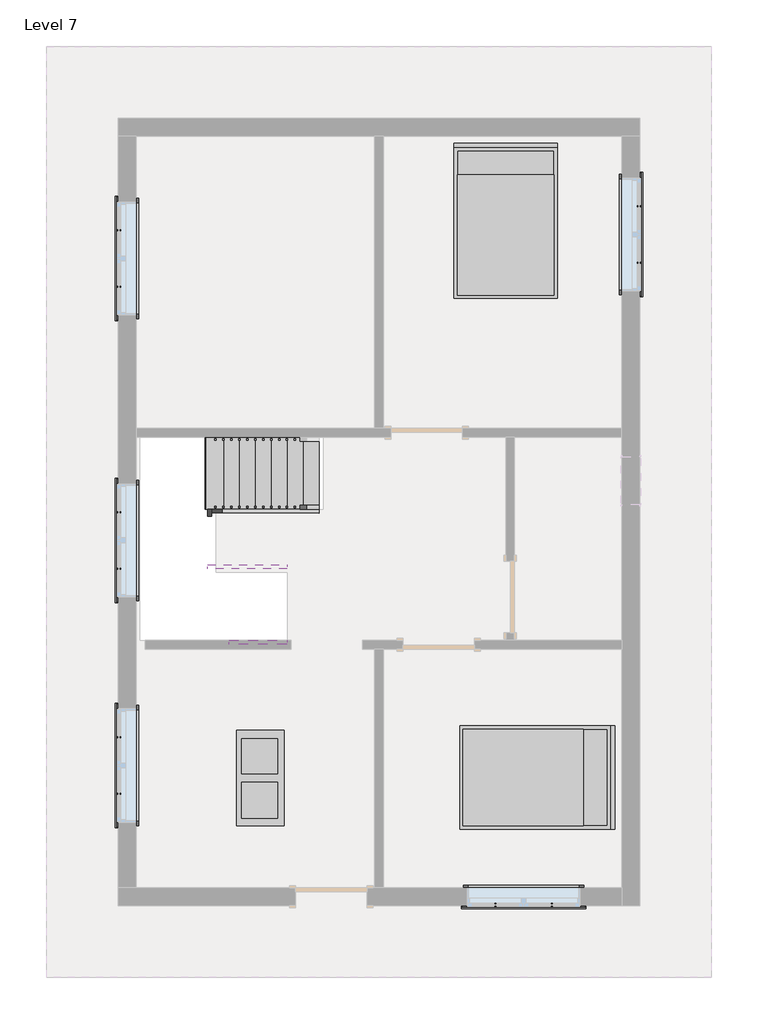
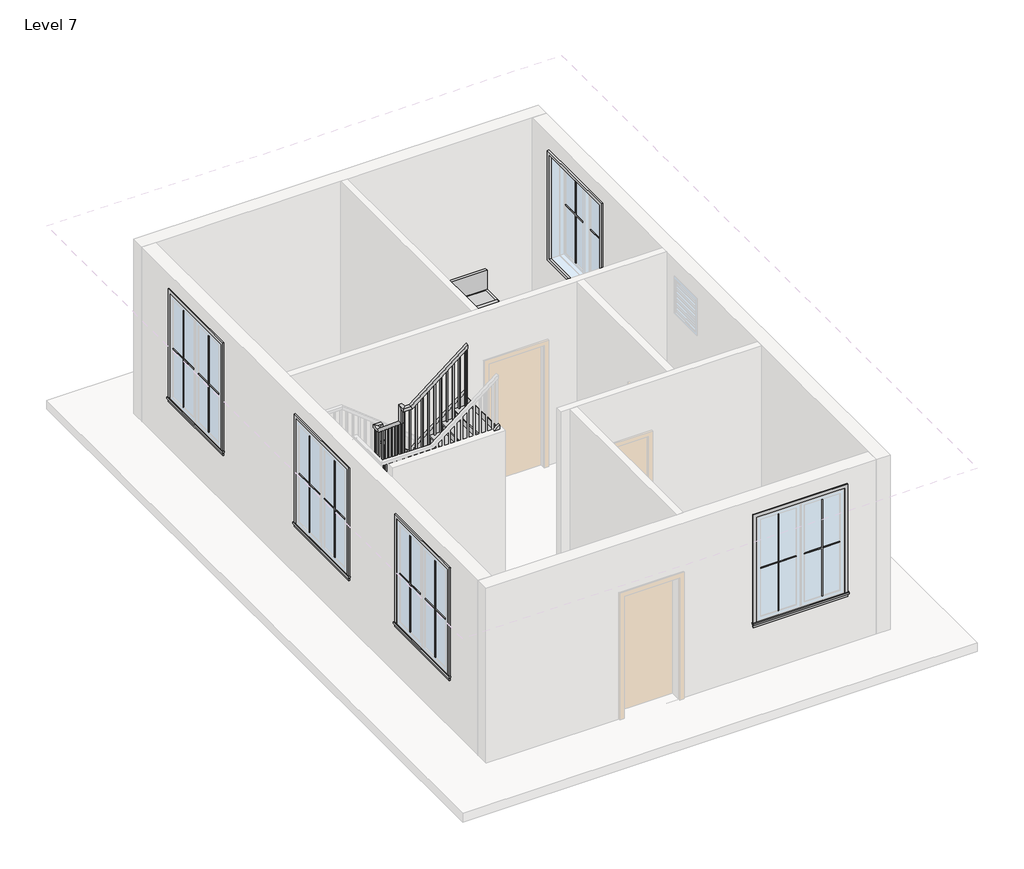
# One storey, part 2 of 2: 21 proxies, 5 members, 2 furniture elements, 1 railing, 1 stair flight.
"""IFC4 building model written with IfcOpenShell, lengths in millimetres."""

from ifc_helpers import new_model, si_unit, frame, origin, place, context, project, spatial, polyline, outline, extrude, faceted_brep, transform, mapped, element, save
from components import muntin_pattern_2x2_muntin_pattern_2x2_bff912c5, muntin_pattern_2x2_muntin_pattern_2x2_c2194282, trim_window_exterior_flat_with_sill_e04b3088, trim_window_interior_flat_picture_frame_2a7685fe, coffee_table_with_brass_mullions_11320_coffee_table_with_5962bef7, bed_17739_bed_17739_15c61121, stair_flight_dc8f8b64

model = new_model("IFC4")

# Units and contexts
model_context = context("Model", 3, world=origin())
ifc_project = project(units=[si_unit("LENGTHUNIT", "METRE", prefix="MILLI")], contexts=[model_context])

# Site, building, storey
site = spatial("IfcSite", under=ifc_project)
building = spatial("IfcBuilding", under=site)
storey = spatial("IfcBuildingStorey", under=building, Name="Level 7", Elevation=16002.0)

# Proxies
placement = place(None, origin())
muntin_pattern_2x2_muntin_pattern_2x2_shape = muntin_pattern_2x2_muntin_pattern_2x2_bff912c5(model_context)
element("IfcBuildingElementProxy", 1, Name="Muntin Pattern_2x2 : Muntin Pattern_2x2", ObjectType="Muntin Pattern_2x2 : Muntin Pattern_2x2", at=placement, inside=storey, context=model_context, shape_type="MappedRepresentation", body=[
    mapped(muntin_pattern_2x2_muntin_pattern_2x2_shape, transform((-626.5715247, -5050.1430046, 16986.25), x_axis=(-1.0, 0.0, 0.0), y_axis=(0.0, -1.0, 0.0), z_axis=(0.0, 0.0, 1.0))),
])
element("IfcBuildingElementProxy", 2, Name="Muntin Pattern_2x2 : Muntin Pattern_2x2", ObjectType="Muntin Pattern_2x2 : Muntin Pattern_2x2", at=placement, inside=storey, context=model_context, shape_type="MappedRepresentation", body=[
    mapped(muntin_pattern_2x2_muntin_pattern_2x2_shape, transform((-6159.0090247, -3629.3305046, 16986.25), x_axis=(0.0, 1.0, 0.0), y_axis=(-1.0, 0.0, 0.0), z_axis=(0.0, 0.0, 1.0))),
])
element("IfcBuildingElementProxy", 3, Name="Muntin Pattern_2x2 : Muntin Pattern_2x2", ObjectType="Muntin Pattern_2x2 : Muntin Pattern_2x2", at=placement, inside=storey, context=model_context, shape_type="MappedRepresentation", body=[
    mapped(muntin_pattern_2x2_muntin_pattern_2x2_shape, transform((489.4409753, 3873.1944954, 16986.25), x_axis=(0.0, -1.0, 0.0), y_axis=(1.0, 0.0, 0.0), z_axis=(0.0, 0.0, 1.0))),
])
element("IfcBuildingElementProxy", 4, Name="Muntin Pattern_2x2 : Muntin Pattern_2x2", ObjectType="Muntin Pattern_2x2 : Muntin Pattern_2x2", at=placement, inside=storey, context=model_context, shape_type="MappedRepresentation", body=[
    mapped(muntin_pattern_2x2_muntin_pattern_2x2_shape, transform((-6159.0090247, 2847.6694954, 16986.25), x_axis=(0.0, 1.0, 0.0), y_axis=(-1.0, 0.0, 0.0), z_axis=(0.0, 0.0, 1.0))),
])
element("IfcBuildingElementProxy", 5, Name="Muntin Pattern_2x2 : Muntin Pattern_2x2", ObjectType="Muntin Pattern_2x2 : Muntin Pattern_2x2", at=placement, inside=storey, context=model_context, shape_type="MappedRepresentation", body=[
    mapped(muntin_pattern_2x2_muntin_pattern_2x2_shape, transform((-6159.0090247, -752.7805046, 16986.25), x_axis=(0.0, 1.0, 0.0), y_axis=(-1.0, 0.0, 0.0), z_axis=(0.0, 0.0, 1.0))),
])
muntin_pattern_2x2_muntin_pattern_2x2_2_shape = muntin_pattern_2x2_muntin_pattern_2x2_c2194282(model_context)
element("IfcBuildingElementProxy", 6, Name="Muntin Pattern_2x2 : Muntin Pattern_2x2", ObjectType="Muntin Pattern_2x2 : Muntin Pattern_2x2", at=placement, inside=storey, context=model_context, shape_type="MappedRepresentation", body=[
    mapped(muntin_pattern_2x2_muntin_pattern_2x2_2_shape, transform((-1347.2965247, -5050.1430046, 16986.25), x_axis=(1.0, 0.0, 0.0), y_axis=(0.0, 1.0, 0.0), z_axis=(0.0, 0.0, 1.0))),
])
element("IfcBuildingElementProxy", 7, Name="Muntin Pattern_2x2 : Muntin Pattern_2x2", ObjectType="Muntin Pattern_2x2 : Muntin Pattern_2x2", at=placement, inside=storey, context=model_context, shape_type="MappedRepresentation", body=[
    mapped(muntin_pattern_2x2_muntin_pattern_2x2_2_shape, transform((-6159.0090247, -2908.6055046, 16986.25), x_axis=(0.0, -1.0, 0.0), y_axis=(1.0, 0.0, 0.0), z_axis=(0.0, 0.0, 1.0))),
])
element("IfcBuildingElementProxy", 8, Name="Muntin Pattern_2x2 : Muntin Pattern_2x2", ObjectType="Muntin Pattern_2x2 : Muntin Pattern_2x2", at=placement, inside=storey, context=model_context, shape_type="MappedRepresentation", body=[
    mapped(muntin_pattern_2x2_muntin_pattern_2x2_2_shape, transform((489.4409753, 3152.4694954, 16986.25), x_axis=(0.0, 1.0, 0.0), y_axis=(-1.0, 0.0, 0.0), z_axis=(0.0, 0.0, 1.0))),
])
element("IfcBuildingElementProxy", 9, Name="Muntin Pattern_2x2 : Muntin Pattern_2x2", ObjectType="Muntin Pattern_2x2 : Muntin Pattern_2x2", at=placement, inside=storey, context=model_context, shape_type="MappedRepresentation", body=[
    mapped(muntin_pattern_2x2_muntin_pattern_2x2_2_shape, transform((-6159.0090247, 3568.3944954, 16986.25), x_axis=(0.0, -1.0, 0.0), y_axis=(1.0, 0.0, 0.0), z_axis=(0.0, 0.0, 1.0))),
])
element("IfcBuildingElementProxy", 10, Name="Muntin Pattern_2x2 : Muntin Pattern_2x2", ObjectType="Muntin Pattern_2x2 : Muntin Pattern_2x2", at=placement, inside=storey, context=model_context, shape_type="MappedRepresentation", body=[
    mapped(muntin_pattern_2x2_muntin_pattern_2x2_2_shape, transform((-6159.0090247, -32.0555046, 16986.25), x_axis=(0.0, -1.0, 0.0), y_axis=(1.0, 0.0, 0.0), z_axis=(0.0, 0.0, 1.0))),
])
trim_window_exterior_flat_with_sill_shape = trim_window_exterior_flat_with_sill_e04b3088(model_context)
element("IfcBuildingElementProxy", 11, Name="Trim-Window-Exterior-Flat : with Sill", ObjectType="Trim-Window-Exterior-Flat : with Sill", at=placement, inside=storey, context=model_context, shape_type="MappedRepresentation", body=[
    mapped(trim_window_exterior_flat_with_sill_shape, transform((-986.9340247, -5059.6680046, 18745.2), x_axis=(1.0, 0.0, 0.0), y_axis=(0.0, 0.0, 1.0), z_axis=(0.0, -1.0, 0.0))),
])
element("IfcBuildingElementProxy", 12, Name="Trim-Window-Exterior-Flat : with Sill", ObjectType="Trim-Window-Exterior-Flat : with Sill", at=placement, inside=storey, context=model_context, shape_type="MappedRepresentation", body=[
    mapped(trim_window_exterior_flat_with_sill_shape, transform((-6168.5340247, -3268.9680046, 18745.2), x_axis=(0.0, -1.0, 0.0), y_axis=(0.0, 0.0, 1.0), z_axis=(-1.0, 0.0, 0.0))),
])
element("IfcBuildingElementProxy", 13, Name="Trim-Window-Exterior-Flat : with Sill", ObjectType="Trim-Window-Exterior-Flat : with Sill", at=placement, inside=storey, context=model_context, shape_type="MappedRepresentation", body=[
    mapped(trim_window_exterior_flat_with_sill_shape, transform((498.9659753, 3512.8319954, 18745.2), x_axis=(0.0, 1.0, 0.0), y_axis=(0.0, 0.0, 1.0), z_axis=(1.0, 0.0, 0.0))),
])
element("IfcBuildingElementProxy", 14, Name="Trim-Window-Exterior-Flat : with Sill", ObjectType="Trim-Window-Exterior-Flat : with Sill", at=placement, inside=storey, context=model_context, shape_type="MappedRepresentation", body=[
    mapped(trim_window_exterior_flat_with_sill_shape, transform((-6168.5340247, 3208.0319954, 18745.2), x_axis=(0.0, -1.0, 0.0), y_axis=(0.0, 0.0, 1.0), z_axis=(-1.0, 0.0, 0.0))),
])
element("IfcBuildingElementProxy", 15, Name="Trim-Window-Exterior-Flat : with Sill", ObjectType="Trim-Window-Exterior-Flat : with Sill", at=placement, inside=storey, context=model_context, shape_type="MappedRepresentation", body=[
    mapped(trim_window_exterior_flat_with_sill_shape, transform((-6168.5340247, -392.4180046, 18745.2), x_axis=(0.0, -1.0, 0.0), y_axis=(0.0, 0.0, 1.0), z_axis=(-1.0, 0.0, 0.0))),
])
trim_window_interior_flat_picture_frame_shape = trim_window_interior_flat_picture_frame_2a7685fe(model_context)
element("IfcBuildingElementProxy", 16, Name="Trim-Window-Interior-Flat : Picture Frame", ObjectType="Trim-Window-Interior-Flat : Picture Frame", at=placement, inside=storey, context=model_context, shape_type="MappedRepresentation", body=[
    mapped(trim_window_interior_flat_picture_frame_shape, transform((-986.9340247, -4831.0680046, 18745.2), x_axis=(-1.0, 0.0, 0.0), y_axis=(0.0, 0.0, 1.0), z_axis=(0.0, 1.0, 0.0))),
])
element("IfcBuildingElementProxy", 17, Name="Trim-Window-Interior-Flat : Picture Frame", ObjectType="Trim-Window-Interior-Flat : Picture Frame", at=placement, inside=storey, context=model_context, shape_type="MappedRepresentation", body=[
    mapped(trim_window_interior_flat_picture_frame_shape, transform((-5939.9340247, -3268.9680046, 18745.2), x_axis=(0.0, 1.0, 0.0), y_axis=(0.0, 0.0, 1.0), z_axis=(1.0, 0.0, 0.0))),
])
element("IfcBuildingElementProxy", 18, Name="Trim-Window-Interior-Flat : Picture Frame", ObjectType="Trim-Window-Interior-Flat : Picture Frame", at=placement, inside=storey, context=model_context, shape_type="MappedRepresentation", body=[
    mapped(trim_window_interior_flat_picture_frame_shape, transform((270.3659753, 3512.8319954, 18745.2), x_axis=(0.0, -1.0, 0.0), y_axis=(0.0, 0.0, 1.0), z_axis=(-1.0, 0.0, 0.0))),
])
element("IfcBuildingElementProxy", 19, Name="Trim-Window-Interior-Flat : Picture Frame", ObjectType="Trim-Window-Interior-Flat : Picture Frame", at=placement, inside=storey, context=model_context, shape_type="MappedRepresentation", body=[
    mapped(trim_window_interior_flat_picture_frame_shape, transform((-5939.9340247, 3208.0319954, 18745.2), x_axis=(0.0, 1.0, 0.0), y_axis=(0.0, 0.0, 1.0), z_axis=(1.0, 0.0, 0.0))),
])
element("IfcBuildingElementProxy", 20, Name="Trim-Window-Interior-Flat : Picture Frame", ObjectType="Trim-Window-Interior-Flat : Picture Frame", at=placement, inside=storey, context=model_context, shape_type="MappedRepresentation", body=[
    mapped(trim_window_interior_flat_picture_frame_shape, transform((-5939.9340247, -392.4180046, 18745.2), x_axis=(0.0, 1.0, 0.0), y_axis=(0.0, 0.0, 1.0), z_axis=(1.0, 0.0, 0.0))),
])
coffee_table_with_brass_mullions_11320_coffee_table_with_shape = coffee_table_with_brass_mullions_11320_coffee_table_with_5962bef7(model_context)
element("IfcBuildingElementProxy", 21, Name="coffee_table_with_brass_mullions_11320 : coffee_table_with_brass_mullions_11320", ObjectType="coffee_table_with_brass_mullions_11320 : coffee_table_with_brass_mullions_11320", at=placement, inside=storey, context=model_context, shape_type="MappedRepresentation", body=[
    mapped(coffee_table_with_brass_mullions_11320_coffee_table_with_shape, transform((-3920.6340247, -2792.7180046, 16002.0), x_axis=(0.0, 1.0, 0.0), y_axis=(-1.0, 0.0, 0.0), z_axis=(0.0, 0.0, 1.0))),
])

# Furniture
bed_17739_bed_17739_shape = bed_17739_bed_17739_15c61121(model_context)
element("IfcFurniture", 22, ObjectType="Bed_17739 : Bed_17739", at=placement, inside=storey, context=model_context, shape_type="MappedRepresentation", body=[
    mapped(bed_17739_bed_17739_shape, transform((-1215.5340247, 3665.2319954, 16002.0), x_axis=(1.0, 0.0, 0.0), y_axis=(0.0, 1.0, 0.0), z_axis=(0.0, 0.0, 1.0))),
])
element("IfcFurniture", 23, ObjectType="Bed_17739 : Bed_17739", at=placement, inside=storey, context=model_context, shape_type="MappedRepresentation", body=[
    mapped(bed_17739_bed_17739_shape, transform((-834.5340247, -3421.3680046, 16002.0), x_axis=(0.0, -1.0, 0.0), y_axis=(1.0, 0.0, 0.0), z_axis=(0.0, 0.0, 1.0))),
])

# Members
element("IfcMember", 24, ObjectType="Stringer - 2\" Width", at=placement, inside=storey, context=model_context, shape_type="SweptSolid", body=[
    extrude(outline(polyline([(16002.0, -3603.1340247), (16233.5686588, -3603.1340247), (17316.4107641, -4974.7340247), (16928.0725136, -4974.7340247), (16002.0, -3801.7088408), (16002.0, -3603.1340247)])), frame((0.0, -43.1680046, 0.0), z_axis=(0.0, 1.0, 0.0), x_axis=(0.0, 0.0, 1.0)), (0.0, 0.0, 1.0), 50.8),
])
element("IfcMember", 25, ObjectType="Stringer - 2\" Width", at=placement, inside=storey, context=model_context, shape_type="SweptSolid", body=[
    extrude(outline(polyline([(7.6319954, 17523.2930346), (7.6319954, 17124.8154064), (-703.5680046, 17723.7206696), (-703.5680046, 18122.1982978), (7.6319954, 17523.2930346)])), frame((-5025.5340247, 0.0, 0.0), z_axis=(1.0, 0.0, 0.0), x_axis=(0.0, 1.0, 0.0)), (0.0, 0.0, 1.0), 50.8),
])
element("IfcMember", 26, ObjectType="Stringer - 2\" Width", at=placement, inside=storey, context=model_context, shape_type="SweptSolid", body=[
    extrude(outline(polyline([(18319.042343, -5025.5340247), (17930.7040926, -5025.5340247), (18732.8093557, -4009.5340247), (19121.1476062, -4009.5340247), (18319.042343, -5025.5340247)])), frame((0.0, -754.3680046, 0.0), z_axis=(0.0, 1.0, 0.0), x_axis=(0.0, 0.0, 1.0)), (0.0, 0.0, 1.0), 50.8),
])
element("IfcMember", 27, ObjectType="Stringer - 2\" Width", at=placement, inside=storey, context=model_context, shape_type="SweptSolid", body=[
    extrude(outline(polyline([(16002.0, -3603.1340247), (16233.5686588, -3603.1340247), (16753.271982, -4261.4249007), (16753.271982, -4753.3200179), (16002.0, -3801.7088408), (16002.0, -3603.1340247)])), frame((0.0, 922.0319954, 0.0), z_axis=(0.0, 1.0, 0.0), x_axis=(0.0, 0.0, 1.0)), (0.0, 0.0, 1.0), 50.8),
])
element("IfcMember", 28, ObjectType="Stringer - 2\" Width", at=placement, inside=storey, context=model_context, shape_type="SweptSolid", body=[
    extrude(outline(polyline([(18536.5206696, -4258.1663605), (18732.8093557, -4009.5340247), (19121.1476062, -4009.5340247), (18536.5206696, -4750.0614777), (18536.5206696, -4258.1663605)])), frame((0.0, -1719.5680046, 0.0), z_axis=(0.0, 1.0, 0.0), x_axis=(0.0, 0.0, 1.0)), (0.0, 0.0, 1.0), 50.8),
])

# Railing
element("IfcRailing", 29, ObjectType="Handrail - Rectangular", at=placement, inside=storey, context=model_context, shape_type="SolidModel", body=[
    faceted_brep([(-3603.1340247, 7.6319954, 17076.8210526), (-3603.1340247, 7.6319954, 17012.0980109), (-3603.1340247, 58.4319954, 17012.0980109), (-3603.1340247, 58.4319954, 17076.8210526), (-4949.3340247, 7.6319954, 18139.6105263), (-5000.1340247, 7.6319954, 18114.9927477), (-5000.1340247, 58.4319954, 18114.9927477), (-4949.3340247, 58.4319954, 18139.6105263), (-4949.3340247, 7.6319954, 18424.3578947), (-5000.1340247, 7.6319954, 18373.5578947), (-5000.1340247, 58.4319954, 18373.5578947), (-4949.3340247, 58.4319954, 18424.3578947), (-5025.5340247, 7.6319954, 18424.3578947), (-5025.5340247, 7.6319954, 18373.5578947), (-5076.3340247, 58.4319954, 18373.5578947), (-5076.3340247, 58.4319954, 18424.3578947), (-5025.5340247, -68.5680046, 18424.3578947), (-5025.5340247, -87.1083685, 18373.5578947), (-5076.3340247, -87.1083685, 18373.5578947), (-5076.3340247, -68.5680046, 18424.3578947), (-5025.5340247, -678.1680046, 18937.7052632), (-5025.5340247, -728.9680046, 18914.0712725), (-5076.3340247, -728.9680046, 18914.0712725), (-5076.3340247, -678.1680046, 18937.7052632), (-5025.5340247, -678.1680046, 19222.4526316), (-5025.5340247, -728.9680046, 19171.6526316), (-5076.3340247, -728.9680046, 19171.6526316), (-5076.3340247, -678.1680046, 19222.4526316), (-5025.5340247, -754.3680046, 19222.4526316), (-5025.5340247, -754.3680046, 19171.6526316), (-5076.3340247, -805.1680046, 19171.6526316), (-5076.3340247, -805.1680046, 19222.4526316), (-4949.3340247, -754.3680046, 19222.4526316), (-4931.6981718, -754.3680046, 19171.6526316), (-4931.6981718, -805.1680046, 19171.6526316), (-4949.3340247, -805.1680046, 19222.4526316), (-4009.5340247, -754.3680046, 19964.4), (-4009.5340247, -805.1680046, 19964.4), (-4009.5340247, -805.1680046, 19899.6769583), (-4009.5340247, -754.3680046, 19899.6769583)], [[[0, 1, 2, 3]], [[1, 0, 4, 5]], [[2, 1, 5, 6]], [[3, 2, 6, 7]], [[0, 3, 7, 4]], [[5, 4, 8, 9]], [[6, 5, 9, 10]], [[7, 6, 10, 11]], [[4, 7, 11, 8]], [[9, 8, 12, 13]], [[10, 9, 13, 14]], [[11, 10, 14, 15]], [[8, 11, 15, 12]], [[13, 12, 16, 17]], [[14, 13, 17, 18]], [[15, 14, 18, 19]], [[12, 15, 19, 16]], [[17, 16, 20, 21]], [[18, 17, 21, 22]], [[19, 18, 22, 23]], [[16, 19, 23, 20]], [[21, 20, 24, 25]], [[22, 21, 25, 26]], [[23, 22, 26, 27]], [[20, 23, 27, 24]], [[25, 24, 28, 29]], [[26, 25, 29, 30]], [[27, 26, 30, 31]], [[24, 27, 31, 28]], [[29, 28, 32, 33]], [[30, 29, 33, 34]], [[31, 30, 34, 35]], [[28, 31, 35, 32]], [[36, 37, 38, 39]], [[33, 32, 36, 39]], [[34, 33, 39, 38]], [[35, 34, 38, 37]], [[32, 35, 37, 36]]]),
    extrude(outline(polyline([(19872.1045898, -4044.4590247), (18889.5789474, -4044.4590247), (18889.5789474, -4025.4090247), (19887.1440635, -4025.4090247), (19872.1045898, -4044.4590247)])), frame((0.0, -789.2930046, 0.0), z_axis=(0.0, 1.0, 0.0), x_axis=(0.0, 0.0, 1.0)), (0.0, 0.0, 1.0), 19.05),
    extrude(outline(polyline([(19791.8940635, -4146.0590247), (18889.5789474, -4146.0590247), (18889.5789474, -4127.0090247), (19806.9335372, -4127.0090247), (19791.8940635, -4146.0590247)])), frame((0.0, -789.2930046, 0.0), z_axis=(0.0, 1.0, 0.0), x_axis=(0.0, 0.0, 1.0)), (0.0, 0.0, 1.0), 19.05),
    extrude(outline(polyline([(19711.6835372, -4247.6590247), (18729.1578947, -4247.6590247), (18729.1578947, -4228.6090247), (19726.7230109, -4228.6090247), (19711.6835372, -4247.6590247)])), frame((0.0, -789.2930046, 0.0), z_axis=(0.0, 1.0, 0.0), x_axis=(0.0, 0.0, 1.0)), (0.0, 0.0, 1.0), 19.05),
    extrude(outline(polyline([(19631.4730109, -4349.2590247), (18729.1578947, -4349.2590247), (18729.1578947, -4330.2090247), (19646.5124846, -4330.2090247), (19631.4730109, -4349.2590247)])), frame((0.0, -789.2930046, 0.0), z_axis=(0.0, 1.0, 0.0), x_axis=(0.0, 0.0, 1.0)), (0.0, 0.0, 1.0), 19.05),
    extrude(outline(polyline([(19551.2624846, -4450.8590247), (18568.7368421, -4450.8590247), (18568.7368421, -4431.8090247), (19566.3019583, -4431.8090247), (19551.2624846, -4450.8590247)])), frame((0.0, -789.2930046, 0.0), z_axis=(0.0, 1.0, 0.0), x_axis=(0.0, 0.0, 1.0)), (0.0, 0.0, 1.0), 19.05),
    extrude(outline(polyline([(19471.0519583, -4552.4590247), (18568.7368421, -4552.4590247), (18568.7368421, -4533.4090247), (19486.0914319, -4533.4090247), (19471.0519583, -4552.4590247)])), frame((0.0, -789.2930046, 0.0), z_axis=(0.0, 1.0, 0.0), x_axis=(0.0, 0.0, 1.0)), (0.0, 0.0, 1.0), 19.05),
    extrude(outline(polyline([(19390.8414319, -4654.0590247), (18408.3157895, -4654.0590247), (18408.3157895, -4635.0090247), (19405.8809056, -4635.0090247), (19390.8414319, -4654.0590247)])), frame((0.0, -789.2930046, 0.0), z_axis=(0.0, 1.0, 0.0), x_axis=(0.0, 0.0, 1.0)), (0.0, 0.0, 1.0), 19.05),
    extrude(outline(polyline([(19310.6309056, -4755.6590247), (18408.3157895, -4755.6590247), (18408.3157895, -4736.6090247), (19325.6703793, -4736.6090247), (19310.6309056, -4755.6590247)])), frame((0.0, -789.2930046, 0.0), z_axis=(0.0, 1.0, 0.0), x_axis=(0.0, 0.0, 1.0)), (0.0, 0.0, 1.0), 19.05),
    extrude(outline(polyline([(19230.4203793, -4857.2590247), (18247.8947368, -4857.2590247), (18247.8947368, -4838.2090247), (19245.459853, -4838.2090247), (19230.4203793, -4857.2590247)])), frame((0.0, -789.2930046, 0.0), z_axis=(0.0, 1.0, 0.0), x_axis=(0.0, 0.0, 1.0)), (0.0, 0.0, 1.0), 19.05),
    extrude(outline(polyline([(19150.209853, -4958.8590247), (18247.8947368, -4958.8590247), (18247.8947368, -4939.8090247), (19165.2493267, -4939.8090247), (19150.209853, -4958.8590247)])), frame((0.0, -789.2930046, 0.0), z_axis=(0.0, 1.0, 0.0), x_axis=(0.0, 0.0, 1.0)), (0.0, 0.0, 1.0), 19.05),
    extrude(outline(polyline([(-668.6430046, 18863.2712725), (-668.6430046, 17927.0526316), (-687.6930046, 17927.0526316), (-687.6930046, 18879.3133778), (-668.6430046, 18863.2712725)])), frame((-5060.4590247, 0.0, 0.0), z_axis=(1.0, 0.0, 0.0), x_axis=(0.0, 1.0, 0.0)), (0.0, 0.0, 1.0), 19.05),
    extrude(outline(polyline([(-567.0430046, 18777.7133778), (-567.0430046, 17927.0526316), (-586.0930046, 17927.0526316), (-586.0930046, 18793.755483), (-567.0430046, 18777.7133778)])), frame((-5060.4590247, 0.0, 0.0), z_axis=(1.0, 0.0, 0.0), x_axis=(0.0, 1.0, 0.0)), (0.0, 0.0, 1.0), 19.05),
    extrude(outline(polyline([(-465.4430046, 18692.155483), (-465.4430046, 17766.6315789), (-484.4930046, 17766.6315789), (-484.4930046, 18708.1975883), (-465.4430046, 18692.155483)])), frame((-5060.4590247, 0.0, 0.0), z_axis=(1.0, 0.0, 0.0), x_axis=(0.0, 1.0, 0.0)), (0.0, 0.0, 1.0), 19.05),
    extrude(outline(polyline([(-363.8430046, 18606.5975883), (-363.8430046, 17766.6315789), (-382.8930046, 17766.6315789), (-382.8930046, 18622.6396935), (-363.8430046, 18606.5975883)])), frame((-5060.4590247, 0.0, 0.0), z_axis=(1.0, 0.0, 0.0), x_axis=(0.0, 1.0, 0.0)), (0.0, 0.0, 1.0), 19.05),
    extrude(outline(polyline([(-262.2430046, 18521.0396935), (-262.2430046, 17606.2105263), (-281.2930046, 17606.2105263), (-281.2930046, 18537.0817988), (-262.2430046, 18521.0396935)])), frame((-5060.4590247, 0.0, 0.0), z_axis=(1.0, 0.0, 0.0), x_axis=(0.0, 1.0, 0.0)), (0.0, 0.0, 1.0), 19.05),
    extrude(outline(polyline([(-160.6430046, 18435.4817988), (-160.6430046, 17606.2105263), (-179.6930046, 17606.2105263), (-179.6930046, 18451.5239041), (-160.6430046, 18435.4817988)])), frame((-5060.4590247, 0.0, 0.0), z_axis=(1.0, 0.0, 0.0), x_axis=(0.0, 1.0, 0.0)), (0.0, 0.0, 1.0), 19.05),
    extrude(outline(polyline([(-59.0430046, 18349.9239041), (-59.0430046, 17445.7894737), (-78.0930046, 17445.7894737), (-78.0930046, 18365.9660093), (-59.0430046, 18349.9239041)])), frame((-5060.4590247, 0.0, 0.0), z_axis=(1.0, 0.0, 0.0), x_axis=(0.0, 1.0, 0.0)), (0.0, 0.0, 1.0), 19.05),
    extrude(outline(polyline([(-5016.0090247, 23.5069954), (-5035.0590247, 23.5069954), (-5035.0590247, 42.5569954), (-5016.0090247, 42.5569954), (-5016.0090247, 23.5069954)])), frame((0.0, 0.0, 17285.3684211), z_axis=(0.0, 0.0, 1.0), x_axis=(1.0, 0.0, 0.0)), (0.0, 0.0, 1.0), 1088.1894737),
    extrude(outline(polyline([(18062.3545898, -4933.4590247), (17124.9473684, -4933.4590247), (17124.9473684, -4914.4090247), (18047.3151161, -4914.4090247), (18062.3545898, -4933.4590247)])), frame((0.0, 23.5069954, 0.0), z_axis=(0.0, 1.0, 0.0), x_axis=(0.0, 0.0, 1.0)), (0.0, 0.0, 1.0), 19.05),
    extrude(outline(polyline([(17982.1440635, -4831.8590247), (17124.9473684, -4831.8590247), (17124.9473684, -4812.8090247), (17967.1045898, -4812.8090247), (17982.1440635, -4831.8590247)])), frame((0.0, 23.5069954, 0.0), z_axis=(0.0, 1.0, 0.0), x_axis=(0.0, 0.0, 1.0)), (0.0, 0.0, 1.0), 19.05),
    extrude(outline(polyline([(17901.9335372, -4730.2590247), (16964.5263158, -4730.2590247), (16964.5263158, -4711.2090247), (17886.8940635, -4711.2090247), (17901.9335372, -4730.2590247)])), frame((0.0, 23.5069954, 0.0), z_axis=(0.0, 1.0, 0.0), x_axis=(0.0, 0.0, 1.0)), (0.0, 0.0, 1.0), 19.05),
    extrude(outline(polyline([(17821.7230109, -4628.6590247), (16964.5263158, -4628.6590247), (16964.5263158, -4609.6090247), (17806.6835372, -4609.6090247), (17821.7230109, -4628.6590247)])), frame((0.0, 23.5069954, 0.0), z_axis=(0.0, 1.0, 0.0), x_axis=(0.0, 0.0, 1.0)), (0.0, 0.0, 1.0), 19.05),
    extrude(outline(polyline([(17741.5124846, -4527.0590247), (16804.1052632, -4527.0590247), (16804.1052632, -4508.0090247), (17726.4730109, -4508.0090247), (17741.5124846, -4527.0590247)])), frame((0.0, 23.5069954, 0.0), z_axis=(0.0, 1.0, 0.0), x_axis=(0.0, 0.0, 1.0)), (0.0, 0.0, 1.0), 19.05),
    extrude(outline(polyline([(17661.3019583, -4425.4590247), (16804.1052632, -4425.4590247), (16804.1052632, -4406.4090247), (17646.2624846, -4406.4090247), (17661.3019583, -4425.4590247)])), frame((0.0, 23.5069954, 0.0), z_axis=(0.0, 1.0, 0.0), x_axis=(0.0, 0.0, 1.0)), (0.0, 0.0, 1.0), 19.05),
    extrude(outline(polyline([(17581.0914319, -4323.8590247), (16643.6842105, -4323.8590247), (16643.6842105, -4304.8090247), (17566.0519583, -4304.8090247), (17581.0914319, -4323.8590247)])), frame((0.0, 23.5069954, 0.0), z_axis=(0.0, 1.0, 0.0), x_axis=(0.0, 0.0, 1.0)), (0.0, 0.0, 1.0), 19.05),
    extrude(outline(polyline([(17500.8809056, -4222.2590247), (16643.6842105, -4222.2590247), (16643.6842105, -4203.2090247), (17485.8414319, -4203.2090247), (17500.8809056, -4222.2590247)])), frame((0.0, 23.5069954, 0.0), z_axis=(0.0, 1.0, 0.0), x_axis=(0.0, 0.0, 1.0)), (0.0, 0.0, 1.0), 19.05),
    extrude(outline(polyline([(17420.6703793, -4120.6590247), (16483.2631579, -4120.6590247), (16483.2631579, -4101.6090247), (17405.6309056, -4101.6090247), (17420.6703793, -4120.6590247)])), frame((0.0, 23.5069954, 0.0), z_axis=(0.0, 1.0, 0.0), x_axis=(0.0, 0.0, 1.0)), (0.0, 0.0, 1.0), 19.05),
    extrude(outline(polyline([(17340.459853, -4019.0590247), (16483.2631579, -4019.0590247), (16483.2631579, -4000.0090247), (17325.4203793, -4000.0090247), (17340.459853, -4019.0590247)])), frame((0.0, 23.5069954, 0.0), z_axis=(0.0, 1.0, 0.0), x_axis=(0.0, 0.0, 1.0)), (0.0, 0.0, 1.0), 19.05),
    extrude(outline(polyline([(17260.2493267, -3917.4590247), (16322.8421053, -3917.4590247), (16322.8421053, -3898.4090247), (17245.209853, -3898.4090247), (17260.2493267, -3917.4590247)])), frame((0.0, 23.5069954, 0.0), z_axis=(0.0, 1.0, 0.0), x_axis=(0.0, 0.0, 1.0)), (0.0, 0.0, 1.0), 19.05),
    extrude(outline(polyline([(17180.0388004, -3815.8590247), (16322.8421053, -3815.8590247), (16322.8421053, -3796.8090247), (17164.9993267, -3796.8090247), (17180.0388004, -3815.8590247)])), frame((0.0, 23.5069954, 0.0), z_axis=(0.0, 1.0, 0.0), x_axis=(0.0, 0.0, 1.0)), (0.0, 0.0, 1.0), 19.05),
    extrude(outline(polyline([(17099.828274, -3714.2590247), (16162.4210526, -3714.2590247), (16162.4210526, -3695.2090247), (17084.7888004, -3695.2090247), (17099.828274, -3714.2590247)])), frame((0.0, 23.5069954, 0.0), z_axis=(0.0, 1.0, 0.0), x_axis=(0.0, 0.0, 1.0)), (0.0, 0.0, 1.0), 19.05),
    extrude(outline(polyline([(-5041.4090247, -770.2430046), (-5041.4090247, -789.2930046), (-5060.4590247, -789.2930046), (-5060.4590247, -770.2430046), (-5041.4090247, -770.2430046)])), frame((0.0, 0.0, 18087.4736842), z_axis=(0.0, 0.0, 1.0), x_axis=(1.0, 0.0, 0.0)), (0.0, 0.0, 1.0), 1084.1789474),
    extrude(outline(polyline([(-5041.4090247, 23.5069954), (-5060.4590247, 23.5069954), (-5060.4590247, 42.5569954), (-5041.4090247, 42.5569954), (-5041.4090247, 23.5069954)])), frame((0.0, 0.0, 17285.3684211), z_axis=(0.0, 0.0, 1.0), x_axis=(1.0, 0.0, 0.0)), (0.0, 0.0, 1.0), 1088.1894737),
    extrude(outline(polyline([(19884.6374846, -4028.5840247), (18889.5789474, -4028.5840247), (18889.5789474, -4009.5340247), (19899.6769583, -4009.5340247), (19884.6374846, -4028.5840247)])), frame((0.0, -789.2930046, 0.0), z_axis=(0.0, 1.0, 0.0), x_axis=(0.0, 0.0, 1.0)), (0.0, 0.0, 1.0), 19.05),
    extrude(outline(polyline([(17027.1374846, -3622.1840247), (16162.4210526, -3622.1840247), (16162.4210526, -3603.1340247), (17012.0980109, -3603.1340247), (17027.1374846, -3622.1840247)])), frame((0.0, 23.5069954, 0.0), z_axis=(0.0, 1.0, 0.0), x_axis=(0.0, 0.0, 1.0)), (0.0, 0.0, 1.0), 19.05),
])

# Stair flight
stair_flight_shape = stair_flight_dc8f8b64(model_context)
element("IfcStairFlight", 30, ObjectType="2\" Tread 1\" Nosing 1/4\" Riser", at=placement, inside=storey, context=model_context, shape_type="MappedRepresentation", body=[
    mapped(stair_flight_shape, transform((0.0, 0.0, 0.0), x_axis=(1.0, 0.0, 0.0), y_axis=(0.0, 1.0, 0.0), z_axis=(0.0, 0.0, 1.0))),
])

save(model, "model.ifc")

# Revit data of these elements
# Type "Muntin Pattern_2x2 : Muntin Pattern_2x2"
#   Width [instance default] = 4' - 0"
#   Thickness = 0' - 0 1/2"
#   Height [instance default] = 4' - 0"
#   Distance = 0' - 0 3/4"
#   Interior Material [instance default] = none
#   Exterior Material [instance default] = none
#   Default Elevation = 0
# Type "Trim-Window-Exterior-Flat : with Sill"
#   Trim Width = 0' - 2 1/4"
#   Trim Thickness_Picture Frame = 0' - 1 1/4"
#   Trim Thickness_with Sill = 0' - 0 3/4"
#   Sill Thickness = 0' - 1 1/4"
#   Opening Width [instance default] = 2' - 0"
#   Opening Height [instance default] = 3' - 0"
#   Default Elevation = 4' - 0"
#   Sill = yes
#   Picture Frame = no
#   Trim Material [instance default] = none
# Type "Trim-Window-Interior-Flat : Picture Frame"
#   Trim Thickness_Picture Frame = 0' - 1 1/4"
#   Trim Width = 0' - 2 1/4"
#   Trim Thickness_with Sill = 0' - 0 3/4"
#   Sill Thickness = 0' - 1 1/4"
#   Opening Width [instance default] = 2' - 0"
#   Opening Height [instance default] = 3' - 0"
#   Default Elevation = 4' - 0"
#   Sill = no
#   Picture Frame = yes
#   Trim Material [instance default] = none
# Type "coffee_table_with_brass_mullions_11320 : coffee_table_with_brass_mullions_11320"
#   Default Elevation = 0
# Type "Bed_17739 : Bed_17739"
#   Default Elevation = 0
# Type "Handrail - Rectangular"
#   Assembly Code = "C2010400"
#   built-in parameter 1008612 = 0.0416667 (stored number, unit not read)
#   built-in parameter 1008611 = 0.0416667 (stored number, unit not read)
#   built-in parameter 1008609 = 0.333333 (stored number, unit not read)
#   built-in parameter 1008604 = 0.166667 (stored number, unit not read)
#   built-in parameter 1008603 = 0.166667 (stored number, unit not read)
#   Railing Height = 3' - 0"
#   built-in parameter 1008630 = 2
#   built-in parameter 1008610 = 2
#   built-in parameter 1008618 = Baluster - Square : 3/4"
# Elements 1, 2, 3, 4, 5, 6, 7, 8, 9, 10 (IfcBuildingElementProxy, "Muntin Pattern_2x2 : Muntin Pattern_2x2")
#   Width = 1' - 11 1/8"
#   Height = 5' - 6 1/2"
#   Interior Material = Wood - Stained
#   Exterior Material = Clad - White
#   Phase Created = New Construction
#   Materials on its faces: "Clad - White", "Wood - Stained"
# Elements 11, 12, 13, 14, 15 (IfcBuildingElementProxy, "Trim-Window-Exterior-Flat : with Sill")
#   Opening Width = 4' - 9"
#   Opening Height = 6' - 0"
#   Trim Material = Clad - White
#   Phase Created = New Construction
#   Materials on its faces: "Clad - White"
# Elements 16, 17, 18, 19, 20 (IfcBuildingElementProxy, "Trim-Window-Interior-Flat : Picture Frame")
#   Opening Width = 4' - 9"
#   Opening Height = 6' - 0"
#   Trim Material = Wood - Stained
#   Phase Created = New Construction
#   Materials on its faces: "Wood - Stained"
# Element 21 (IfcBuildingElementProxy, "coffee_table_with_brass_mullions_11320 : coffee_table_with_brass_mullions_11320")
#   Phase Created = New Construction
#   Materials on its faces: "Default Wall", "TABLE", "Glass", "Default"
# Elements 22, 23 (IfcFurniture, "Bed_17739 : Bed_17739")
#   Phase Created = New Construction
#   Materials on its faces: "legs", "sheets", "bed frame", "Blanket"
# Elements 24, 25, 26, 27, 28 (IfcMember, "Stringer - 2\" Width")
#   Phase Created = New Construction
# Element 29 (IfcRailing, "Handrail - Rectangular")
#   Phase Created = New Construction
#   Materials on its faces: "Oak Flooring"
# Element 30 (IfcStairFlight, "2\" Tread 1\" Nosing 1/4\" Riser")
#   Phase Created = New Construction
# Materials
#   "Clad - White": class "Wood", colour RGB 242 242 238, transparency 0, Cost = 0
#   "Wood - Stained": class "Wood", colour RGB 224 178 126, transparency 0, Cost = 0
#   "Default Wall": colour RGB 128 128 128, transparency 0, Cost = 0
#   "TABLE": class "Generic", colour RGB 120 120 120, transparency 0, Cost = 0
#   "Glass": class "Glass", colour RGB 0 128 192, transparency 0.75, Description = "Soda Lime Glass", Cost = 0
#   "Default": colour RGB 127 127 127, transparency 0, Cost = 0
#   "legs": colour RGB 90 73 37, transparency 0, Cost = 0
#   "sheets": colour RGB 200 195 176, transparency 0, Cost = 0
#   "bed frame": colour RGB 90 73 37, transparency 0, Cost = 0
#   "Blanket": class "System", colour RGB 59 0 1, transparency 0, Cost = 0
#   "Oak Flooring": class "Wood", colour RGB 216 169 114, transparency 0, Description = "Quercus Rubra", Cost = 0
